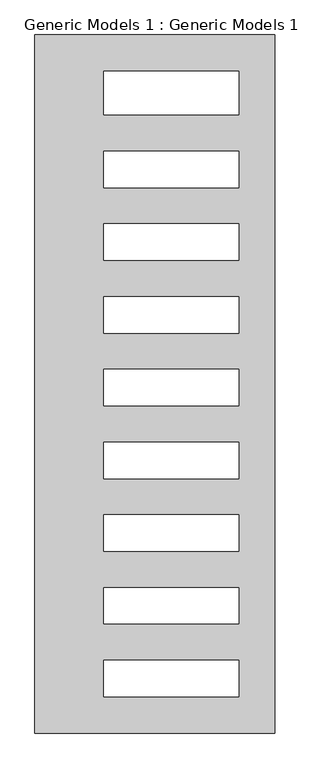
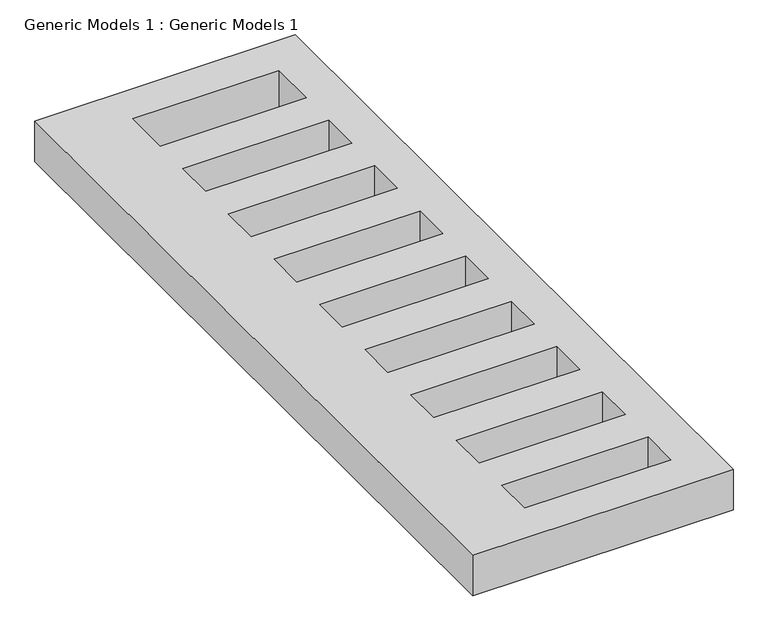
"""IFC4 building model written with IfcOpenShell, lengths in millimetres: proxy geometry, Generic Models 1 : Generic Models 1."""

from ifc_helpers import new_model, si_unit, frame, origin, place, context, project, spatial, polyline, outline, extrude, source, transform, mapped, element, save


def generic_models_1_generic_models_1_b1455ff5(model_context):
    return source(origin(), model_context, "Body", "SweptSolid", [
        extrude(outline(polyline([(-7804.5025595, 1580.5132107), (-7804.5025595, -3296.2867893), (-9480.9025595, -3296.2867893), (-9480.9025595, 1580.5132107), (-7804.5025595, 1580.5132107)]), holes=[polyline([(-8998.3025595, 1326.5132107), (-8998.3025595, 1021.7132107), (-8058.5025595, 1021.7132107), (-8058.5025595, 1326.5132107), (-8998.3025595, 1326.5132107)]), polyline([(-8058.5025595, -2788.2867893), (-8998.3025595, -2788.2867893), (-8998.3025595, -3042.2867893), (-8058.5025595, -3042.2867893), (-8058.5025595, -2788.2867893)]), polyline([(-8998.3025595, 767.7132107), (-8998.3025595, 513.7132107), (-8058.5025595, 513.7132107), (-8058.5025595, 767.7132107), (-8998.3025595, 767.7132107)]), polyline([(-8998.3025595, 259.7132107), (-8998.3025595, 5.7132107), (-8058.5025595, 5.7132107), (-8058.5025595, 259.7132107), (-8998.3025595, 259.7132107)]), polyline([(-8998.3025595, -248.2867893), (-8998.3025595, -502.2867893), (-8058.5025595, -502.2867893), (-8058.5025595, -248.2867893), (-8998.3025595, -248.2867893)]), polyline([(-8998.3025595, -756.2867893), (-8998.3025595, -1010.2867893), (-8058.5025595, -1010.2867893), (-8058.5025595, -756.2867893), (-8998.3025595, -756.2867893)]), polyline([(-8998.3025595, -1264.2867893), (-8998.3025595, -1518.2867893), (-8058.5025595, -1518.2867893), (-8058.5025595, -1264.2867893), (-8998.3025595, -1264.2867893)]), polyline([(-8998.3025595, -1772.2867893), (-8998.3025595, -2026.2867893), (-8058.5025595, -2026.2867893), (-8058.5025595, -1772.2867893), (-8998.3025595, -1772.2867893)]), polyline([(-8998.3025595, -2280.2867893), (-8998.3025595, -2534.2867893), (-8058.5025595, -2534.2867893), (-8058.5025595, -2280.2867893), (-8998.3025595, -2280.2867893)])]), frame((0.0, 0.0, 2925.0), z_axis=(0.0, 0.0, 1.0), x_axis=(1.0, 0.0, 0.0)), (0.0, 0.0, 1.0), 275.4),
    ])


if __name__ == "__main__":
    model = new_model("IFC4")
    model_context = context("Model", 3, world=origin())
    ifc_project = project(units=[si_unit("LENGTHUNIT", "METRE", prefix="MILLI")], contexts=[model_context])
    site = spatial("IfcSite", under=ifc_project)
    building = spatial("IfcBuilding", under=site)
    placement = place(None, origin())
    generic_models_1_generic_models_1_shape = generic_models_1_generic_models_1_b1455ff5(model_context)
    element("IfcBuildingElementProxy", 1, Name="Generic Models 1 : Generic Models 1", ObjectType="Generic Models 1 : Generic Models 1", at=placement, inside=building, context=model_context, shape_type="MappedRepresentation", body=[
        mapped(generic_models_1_generic_models_1_shape, transform((0.0, 0.0, 0.0), x_axis=(1.0, 0.0, 0.0), y_axis=(0.0, 1.0, 0.0), z_axis=(0.0, 0.0, 1.0))),
    ])
    save(model, "model.ifc")
